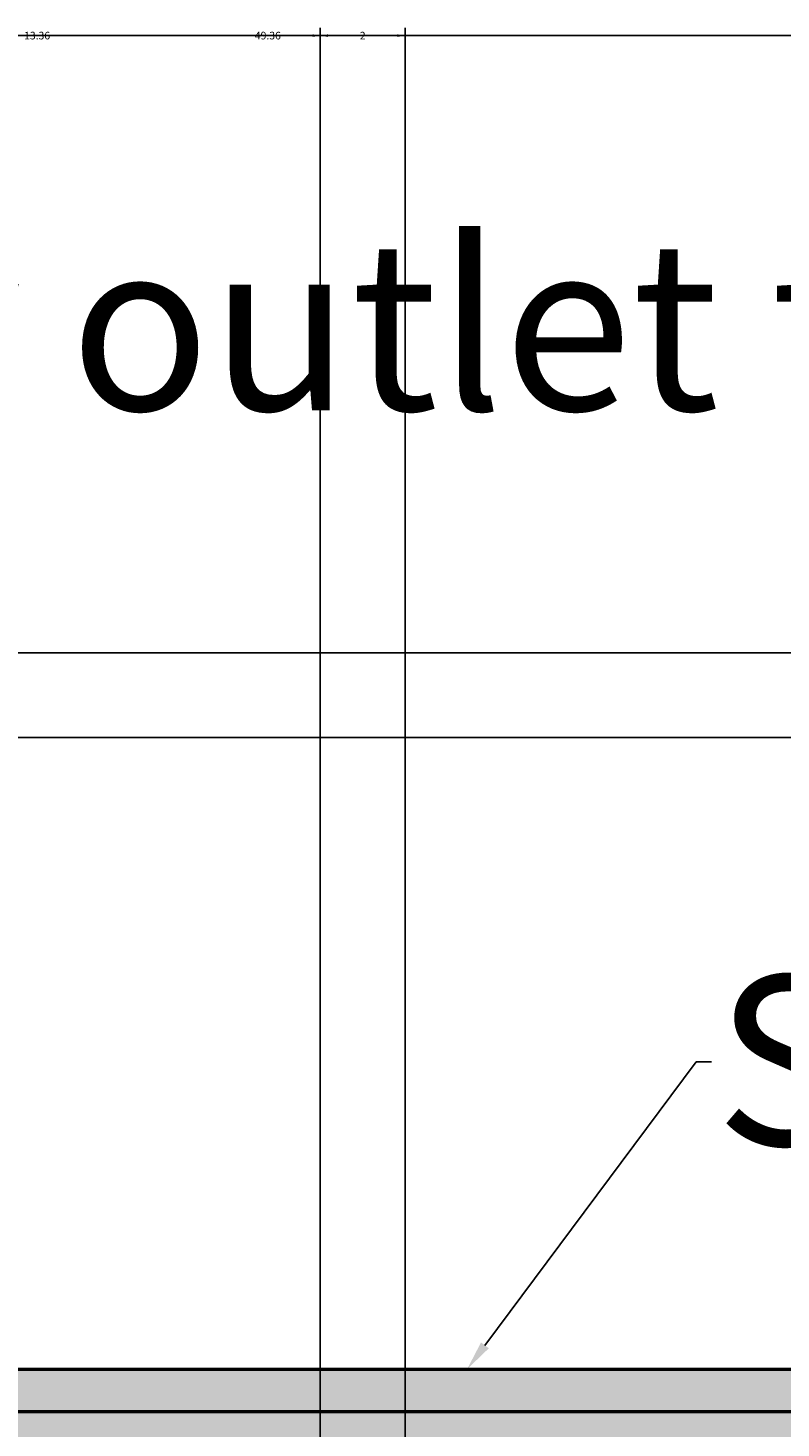
# Model space of a CAD drawing. Units: inches. Extents: x -12 to 334, y -10 to 186.
# Tile 68 of 77: x 239 to 257, y 137 to 170. Entities that reach past the tile are written whole.
import ezdxf
from ezdxf import colors
from ezdxf.entities.mleader import LeaderData, LeaderLine
from ezdxf.math import Vec2, Vec3

# ---------------------------------------------------------------- set-up
doc = ezdxf.new("R2010")
doc.units = ezdxf.units.IN
doc.header["$MEASUREMENT"] = 0
for name, color, linetype, lineweight in [('M-ANNO-TEXT', 3, 'Continuous', 25), ('M-DIMS', 2, 'Continuous', 18), ('M-EQPM', 7, 'Continuous', 50), ('M-EQPM-PATT', 8, 'Continuous', 18)]:
    doc.layers.add(name, color=color, linetype=linetype, lineweight=lineweight)
doc.styles.get("Standard").update_dxf_attribs({"font": 'arial.ttf'})
doc.dimstyles.get("Standard").update_dxf_attribs({"dimtxt": 0.18, "dimasz": 0.18, "dimexe": 0.18, "dimexo": 0.0625, "dimgap": 0.09, "dimtad": 0, "dimtih": 1, "dimtoh": 1, "dimdec": 4, "dimzin": 0, "dimdsep": 46, "dimtxsty": 'Standard', "dimcen": 0.09, "dimadec": 0, "dimazin": 0, "dimtfac": 1, "dimtdec": 4, "dimtofl": 0, "dimtmove": 0, "dimatfit": 3, "dimfxl": 1, "dimtolj": 1, "dimtzin": 0, "dimarcsym": 0})

# ---------------------------------------------------------------- blocks, each defined once
blk = doc.blocks.new('*D21')
at = {"layer": 'Defpoints', "color": 0, "transparency": 16777216}
for p in [(269.381, 169.385), (220.017, 154.835), (269.381, 137.943)]:
    blk.add_point(p, dxfattribs=at)
at = {"layer": 'M-DIMS', "color": 0, "lineweight": -2, "transparency": 16777216}
for p, q in [((220.017, 154.897), (220.017, 169.565)), ((220.197, 169.385), (244.301, 169.385)), ((269.201, 169.385), (245.096, 169.385)), ((269.381, 138.006), (269.381, 169.565))]:
    blk.add_line(p, q, dxfattribs=at)
at = {"layer": 'M-DIMS', "color": 0, "transparency": 16777216}
for points in [[(220.197, 169.415), (220.197, 169.355), (220.017, 169.385)], [(269.201, 169.415), (269.201, 169.355), (269.381, 169.385)]]:
    blk.add_solid(points, dxfattribs=at)
at = {"layer": 'M-DIMS', "color": 0, "transparency": 16777216, "insert": (244.699, 169.385), "char_height": 0.18, "attachment_point": 5}
blk.add_mtext('\\A1;49.36', dxfattribs=at)
blk = doc.blocks.new('*D23')
at = {"layer": 'Defpoints', "color": 0, "transparency": 16777216}
for p in [(220.017, 154.835), (220.017, 152.835), (295.976, 152.835)]:
    blk.add_point(p, dxfattribs=at)
at = {"layer": 'M-DIMS', "color": 0, "lineweight": -2, "transparency": 16777216}
for p, q in [((220.079, 154.835), (296.156, 154.835)), ((295.976, 154.655), (295.976, 154.015)), ((295.976, 153.015), (295.976, 153.654)), ((220.079, 152.835), (296.156, 152.835))]:
    blk.add_line(p, q, dxfattribs=at)
at = {"layer": 'M-DIMS', "color": 0, "transparency": 16777216}
for points in [[(295.946, 154.655), (296.006, 154.655), (295.976, 154.835)], [(295.946, 153.015), (296.006, 153.015), (295.976, 152.835)]]:
    blk.add_solid(points, dxfattribs=at)
at = {"layer": 'M-DIMS', "color": 0, "transparency": 16777216, "insert": (295.976, 153.835), "char_height": 0.18, "attachment_point": 5}
blk.add_mtext('\\A1;2', dxfattribs=at)
blk = doc.blocks.new('*D36')
at = {"layer": 'Defpoints', "color": 0, "transparency": 16777216}
for p in [(247.935, 169.385), (245.935, 82.697), (247.935, 82.697)]:
    blk.add_point(p, dxfattribs=at)
at = {"layer": 'M-DIMS', "color": 0, "lineweight": -2, "transparency": 16777216}
for p, q in [((245.935, 82.759), (245.935, 169.565)), ((246.115, 169.385), (246.786, 169.385)), ((247.755, 169.385), (247.085, 169.385)), ((247.935, 82.759), (247.935, 169.565))]:
    blk.add_line(p, q, dxfattribs=at)
at = {"layer": 'M-DIMS', "color": 0, "transparency": 16777216}
for points in [[(246.115, 169.415), (246.115, 169.355), (245.935, 169.385)], [(247.755, 169.415), (247.755, 169.355), (247.935, 169.385)]]:
    blk.add_solid(points, dxfattribs=at)
at = {"layer": 'M-DIMS', "color": 0, "transparency": 16777216, "insert": (246.935, 169.385), "char_height": 0.18, "attachment_point": 5}
blk.add_mtext('\\A1;2', dxfattribs=at)
blk = doc.blocks.new('*D37')
at = {"layer": 'Defpoints', "color": 0, "transparency": 16777216}
for p in [(245.935, 169.385), (232.576, 46.854), (245.935, 46.854)]:
    blk.add_point(p, dxfattribs=at)
at = {"layer": 'M-DIMS', "color": 0, "lineweight": -2, "transparency": 16777216}
for p, q in [((232.576, 46.917), (232.576, 169.565)), ((232.756, 169.385), (238.871, 169.385)), ((245.755, 169.385), (239.641, 169.385)), ((245.935, 46.917), (245.935, 169.565))]:
    blk.add_line(p, q, dxfattribs=at)
at = {"layer": 'M-DIMS', "color": 0, "transparency": 16777216}
for points in [[(232.756, 169.415), (232.756, 169.355), (232.576, 169.385)], [(245.755, 169.415), (245.755, 169.355), (245.935, 169.385)]]:
    blk.add_solid(points, dxfattribs=at)
at = {"layer": 'M-DIMS', "color": 0, "transparency": 16777216, "insert": (239.256, 169.385), "char_height": 0.18, "attachment_point": 5}
blk.add_mtext('\\A1;13.36', dxfattribs=at)

msp = doc.modelspace()

# ---------------------------------------------------------------- hatches: boundary and pattern name
at = {"layer": 'M-EQPM-PATT', "transparency": 33554556}
h = msp.add_hatch(color=256, dxfattribs=at)
h.set_gradient(color1=(248, 206, 179), color2=(248, 206, 179), tint=1)
h.paths.add_polyline_path([(179.7818, 136.8871), (126.9567, 136.8871), (106.1771, 100.8958), (171.5458, 100.8958)])
h.paths.add_polyline_path([(268.3808, 136.9435), (214.0166, 136.9435), (214.0166, 154.8345), (196.3421, 154.8345), (196.3421, 136.8871), (179.7818, 136.8871), (171.5458, 100.8958), (231.7758, 100.8958, -0.4142136), (251.9801, 80.6915), (279.7263, 80.6915, 0.1631825)])
at = {"layer": 'M-EQPM-PATT'}
h = msp.add_hatch(color=256, dxfattribs=at)
h.set_gradient(color1=(99, 100, 102), color2=(99, 100, 102), tint=1)
h.paths.add_polyline_path([(126.9567, 136.8871), (179.7818, 136.8871), (180.0106, 137.8871), (126.3793, 137.8871), (106.1771, 102.8958), (86.8879, 102.8958), (86.8879, 109.0583), (84.7229, 109.0583), (84.7229, 100.8958), (106.1771, 100.8958)])
h.paths.add_polyline_path([(196.3421, 152.8345), (195.3421, 152.8345), (195.3421, 137.8871), (180.0106, 137.8871), (179.7818, 136.8871), (196.3421, 136.8871)])
h.paths.add_polyline_path([(215.0166, 152.8345), (214.0166, 152.8345), (214.0166, 136.9435), (268.3808, 136.9435, -0.2673785), (268.3808, 46.8541), (249.3759, 46.8541), (249.8485, 45.8541), (269.3808, 45.8541, 0.2615891), (269.3808, 137.9435), (215.0166, 137.9435)])

# ---------------------------------------------------------------- linework, layer by layer
at = {"layer": 'M-EQPM'}
for points in [[(214.0166, 154.8345), (214.0166, 136.9435), (268.3808, 136.9435)], [(215.0166, 152.8345), (215.0166, 137.9435), (269.3808, 137.9435)]]:
    msp.add_lwpolyline(points, dxfattribs=at)

# ---------------------------------------------------------------- dimensions: what is measured, and where the dimension line sits
at = {"layer": 'M-DIMS'}
for base, p1, p2, override, picture, middle in [((269.3808, 169.3845), (220.0166, 154.8345), (269.3808, 137.9435), {"dimdec": 2, "dimlfac": 1, "dimrnd": 0, "dimzin": 0, "dimdsep": 46, "dimlunit": 2}, '*D21', (244.6987, 169.3845)), ((245.9354, 169.3845), (232.5761, 46.8541), (245.9354, 46.8541), {"dimdec": 2, "dimlfac": 1, "dimrnd": 0, "dimzin": 0, "dimdsep": 46, "dimlunit": 2}, '*D37', (239.2558, 169.3845)), ((247.9354, 169.3845), (245.9354, 82.6969), (247.9354, 82.6969), {"dimdec": 0, "dimlfac": 1, "dimrnd": 0, "dimzin": 0, "dimdsep": 46, "dimlunit": 2}, '*D36', (246.9354, 169.3845))]:
    dim = msp.add_linear_dim(base=base, p1=p1, p2=p2, dimstyle='Standard', override=override, dxfattribs=at)
    dim.commit()
    dim.dimension.update_dxf_attribs({"geometry": picture, "text_midpoint": middle})
dim = msp.add_linear_dim(base=(295.9756, 152.8345), p1=(220.0166, 154.8345), p2=(220.0166, 152.8345), angle=90, dimstyle='Standard', override={"dimdec": 0, "dimlfac": 1, "dimrnd": 0, "dimzin": 0, "dimdsep": 46, "dimlunit": 2}, dxfattribs=at)
dim.commit()
dim.dimension.update_dxf_attribs({"geometry": '*D23', "text_midpoint": (295.9756, 153.8345)})

# ---------------------------------------------------------------- leaders
at = {"layer": 'M-ANNO-TEXT'}
ml = msp.add_multileader_mtext('Standard', dxfattribs=at)
ml.set_content('vapour outlet to column', color=256)
ml.set_leader_properties()
ml.build(insert=Vec2(0, 0))
ml.multileader.update_dxf_attribs({"dogleg_length": 0.36, "arrow_head_size": 0.7})
ctx = ml.context
ctx.base_point, ctx.arrow_head_size, ctx.landing_gap_size, ctx.plane_origin = Vec3(220.6842, 161.9963), 0.7, 0.09, Vec3(211.0929, 154.8345)
notes = []
notes.append((ctx, [(0, (1, 1, 0), (215.2277, 161.9963), (1, 0), 5.4565, [(0, [(211.0929, 154.8345)], 0, [])])]))
ctx.mtext.insert, ctx.mtext.flow_direction = Vec3(220.7742, 164.5515), 5
ml = msp.add_multileader_mtext('Standard', dxfattribs=at)
ml.set_content('Shell', color=256)
ml.set_leader_properties()
ml.build(insert=Vec2(0, 0))
ml.multileader.update_dxf_attribs({"dogleg_length": 0.36, "arrow_head_size": 0.7})
ctx = ml.context
ctx.base_point, ctx.arrow_head_size, ctx.landing_gap_size, ctx.plane_origin = Vec3(255.1635, 145.1886), 0.7, 0.09, Vec3(249.4005, 137.9435)
notes.append((ctx, [(0, (1, 1, 0), (254.8035, 145.1886), (1, 0), 0.36, [(0, [(249.4005, 137.9435)], 0, [])])]))
ctx.mtext.insert, ctx.mtext.flow_direction = Vec3(255.2535, 147.2227), 5
for ctx, leaders in notes:
    for number, flags, end, landing, length, lines in leaders:
        leader = LeaderData()
        leader.index, (leader.has_last_leader_line, leader.has_dogleg_vector, leader.attachment_direction) = number, flags
        leader.last_leader_point, leader.dogleg_vector, leader.dogleg_length = Vec3(end), Vec3(landing), length
        for number, points, colour, breaks in lines:
            line = LeaderLine()
            line.index, line.vertices, line.color, line.breaks = number, Vec3.list(points), colors.encode_raw_color(colour), breaks
            leader.lines.append(line)
        ctx.leaders.append(leader)

doc.saveas('drawing.dxf')
